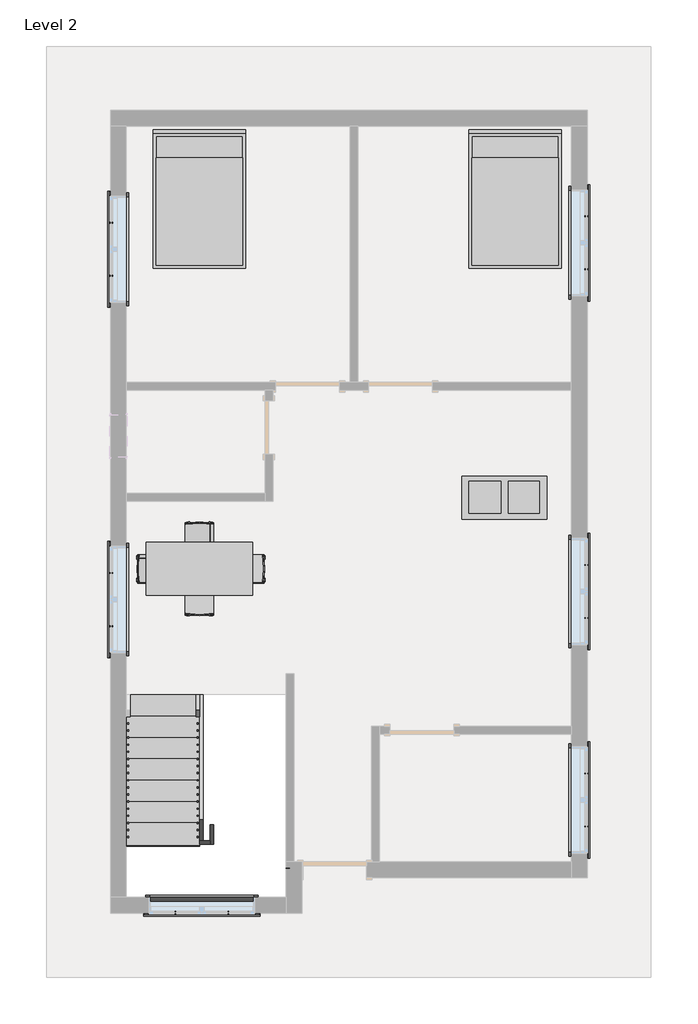
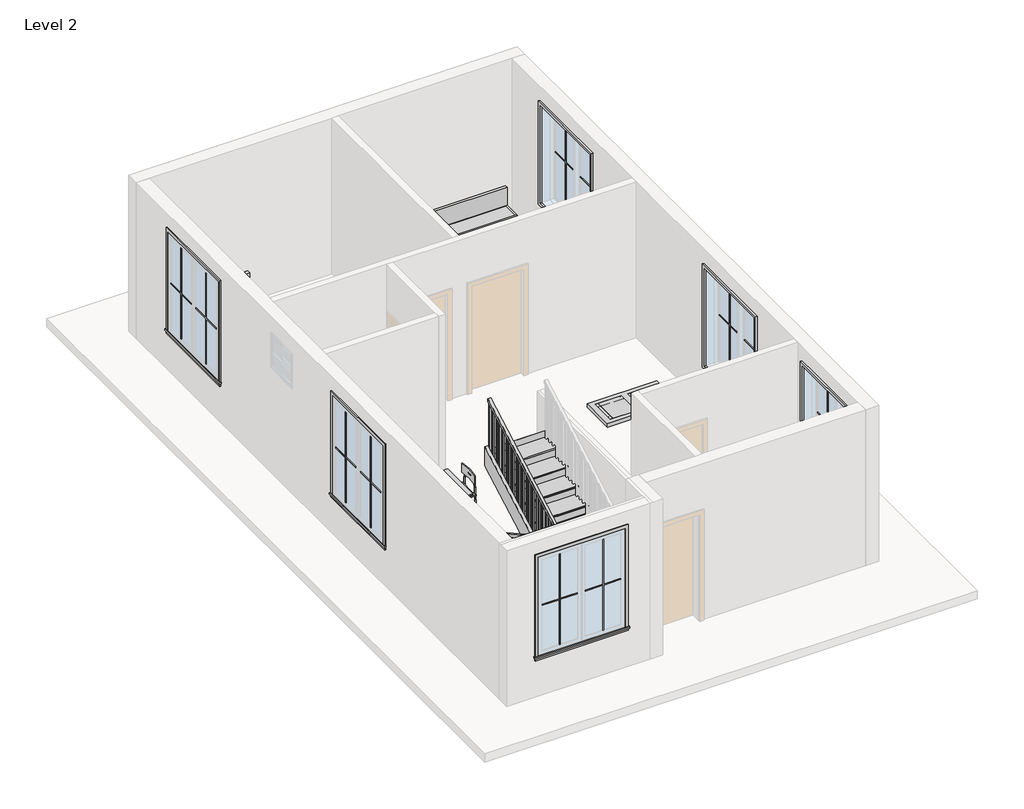
# One storey, part 3 of 3: 25 proxies, 6 members, 3 furniture elements, 1 railing, 1 stair flight.
"""IFC4 building model written with IfcOpenShell, lengths in millimetres."""

from ifc_helpers import new_model, si_unit, frame, origin, place, context, project, spatial, polyline, outline, extrude, faceted_brep, transform, mapped, element, save
from components import muntin_pattern_2x2_muntin_pattern_2x2_f6a80940, muntin_pattern_2x2_muntin_pattern_2x2_09b00a1c, trim_window_exterior_flat_with_sill_698ed857, trim_window_interior_flat_picture_frame_92551a5e, coffee_table_with_brass_mullions_11320_coffee_table_with_5962bef7, bed_17739_bed_17739_15c61121, dining_table_w_chairs_11374_0cdfc61b, stair_flight_d5b1d6b9

model = new_model("IFC4")

# Units and contexts
model_context = context("Model", 3, world=origin())
ifc_project = project(units=[si_unit("LENGTHUNIT", "METRE", prefix="MILLI")], contexts=[model_context])

# Site, building, storey
site = spatial("IfcSite", under=ifc_project)
building = spatial("IfcBuilding", under=site)
storey = spatial("IfcBuildingStorey", under=building, Name="Level 2", Elevation=3048.0)

# Proxies
placement = place(None, origin())
muntin_pattern_2x2_muntin_pattern_2x2_shape = muntin_pattern_2x2_muntin_pattern_2x2_f6a80940(model_context)
element("IfcBuildingElementProxy", 1, Name="Muntin Pattern_2x2 : Muntin Pattern_2x2", ObjectType="Muntin Pattern_2x2 : Muntin Pattern_2x2", at=placement, inside=storey, context=model_context, shape_type="MappedRepresentation", body=[
    mapped(muntin_pattern_2x2_muntin_pattern_2x2_shape, transform((-2773.368364, -6686.2830018, 4032.25), x_axis=(-1.0, 0.0, 0.0), y_axis=(0.0, -1.0, 0.0), z_axis=(0.0, 0.0, 1.0))),
])
element("IfcBuildingElementProxy", 2, Name="Muntin Pattern_2x2 : Muntin Pattern_2x2", ObjectType="Muntin Pattern_2x2 : Muntin Pattern_2x2", at=placement, inside=storey, context=model_context, shape_type="MappedRepresentation", body=[
    mapped(muntin_pattern_2x2_muntin_pattern_2x2_shape, transform((2349.494136, -4693.9705018, 4032.25), x_axis=(0.0, -1.0, 0.0), y_axis=(1.0, 0.0, 0.0), z_axis=(0.0, 0.0, 1.0))),
])
element("IfcBuildingElementProxy", 3, Name="Muntin Pattern_2x2 : Muntin Pattern_2x2", ObjectType="Muntin Pattern_2x2 : Muntin Pattern_2x2", at=placement, inside=storey, context=model_context, shape_type="MappedRepresentation", body=[
    mapped(muntin_pattern_2x2_muntin_pattern_2x2_shape, transform((2349.494136, -1712.6455018, 4032.25), x_axis=(0.0, -1.0, 0.0), y_axis=(1.0, 0.0, 0.0), z_axis=(0.0, 0.0, 1.0))),
])
element("IfcBuildingElementProxy", 4, Name="Muntin Pattern_2x2 : Muntin Pattern_2x2", ObjectType="Muntin Pattern_2x2 : Muntin Pattern_2x2", at=placement, inside=storey, context=model_context, shape_type="MappedRepresentation", body=[
    mapped(muntin_pattern_2x2_muntin_pattern_2x2_shape, transform((-4451.355864, -2586.5525081, 4032.25), x_axis=(0.0, 1.0, 0.0), y_axis=(-1.0, 0.0, 0.0), z_axis=(0.0, 0.0, 1.0))),
])
element("IfcBuildingElementProxy", 5, Name="Muntin Pattern_2x2 : Muntin Pattern_2x2", ObjectType="Muntin Pattern_2x2 : Muntin Pattern_2x2", at=placement, inside=storey, context=model_context, shape_type="MappedRepresentation", body=[
    mapped(muntin_pattern_2x2_muntin_pattern_2x2_shape, transform((2349.494136, 3272.1044982, 4032.25), x_axis=(0.0, -1.0, 0.0), y_axis=(1.0, 0.0, 0.0), z_axis=(0.0, 0.0, 1.0))),
])
element("IfcBuildingElementProxy", 6, Name="Muntin Pattern_2x2 : Muntin Pattern_2x2", ObjectType="Muntin Pattern_2x2 : Muntin Pattern_2x2", at=placement, inside=storey, context=model_context, shape_type="MappedRepresentation", body=[
    mapped(muntin_pattern_2x2_muntin_pattern_2x2_shape, transform((-4451.355864, 2421.2162133, 4032.25), x_axis=(0.0, 1.0, 0.0), y_axis=(-1.0, 0.0, 0.0), z_axis=(0.0, 0.0, 1.0))),
])
muntin_pattern_2x2_muntin_pattern_2x2_2_shape = muntin_pattern_2x2_muntin_pattern_2x2_09b00a1c(model_context)
element("IfcBuildingElementProxy", 7, Name="Muntin Pattern_2x2 : Muntin Pattern_2x2", ObjectType="Muntin Pattern_2x2 : Muntin Pattern_2x2", at=placement, inside=storey, context=model_context, shape_type="MappedRepresentation", body=[
    mapped(muntin_pattern_2x2_muntin_pattern_2x2_2_shape, transform((-3532.193364, -6686.2830018, 4032.25), x_axis=(1.0, 0.0, 0.0), y_axis=(0.0, 1.0, 0.0), z_axis=(0.0, 0.0, 1.0))),
])
element("IfcBuildingElementProxy", 8, Name="Muntin Pattern_2x2 : Muntin Pattern_2x2", ObjectType="Muntin Pattern_2x2 : Muntin Pattern_2x2", at=placement, inside=storey, context=model_context, shape_type="MappedRepresentation", body=[
    mapped(muntin_pattern_2x2_muntin_pattern_2x2_2_shape, transform((2349.494136, -5452.7955018, 4032.25), x_axis=(0.0, 1.0, 0.0), y_axis=(-1.0, 0.0, 0.0), z_axis=(0.0, 0.0, 1.0))),
])
element("IfcBuildingElementProxy", 9, Name="Muntin Pattern_2x2 : Muntin Pattern_2x2", ObjectType="Muntin Pattern_2x2 : Muntin Pattern_2x2", at=placement, inside=storey, context=model_context, shape_type="MappedRepresentation", body=[
    mapped(muntin_pattern_2x2_muntin_pattern_2x2_2_shape, transform((2349.494136, -2471.4705018, 4032.25), x_axis=(0.0, 1.0, 0.0), y_axis=(-1.0, 0.0, 0.0), z_axis=(0.0, 0.0, 1.0))),
])
element("IfcBuildingElementProxy", 10, Name="Muntin Pattern_2x2 : Muntin Pattern_2x2", ObjectType="Muntin Pattern_2x2 : Muntin Pattern_2x2", at=placement, inside=storey, context=model_context, shape_type="MappedRepresentation", body=[
    mapped(muntin_pattern_2x2_muntin_pattern_2x2_2_shape, transform((-4451.355864, -1827.7275081, 4032.25), x_axis=(0.0, -1.0, 0.0), y_axis=(1.0, 0.0, 0.0), z_axis=(0.0, 0.0, 1.0))),
])
element("IfcBuildingElementProxy", 11, Name="Muntin Pattern_2x2 : Muntin Pattern_2x2", ObjectType="Muntin Pattern_2x2 : Muntin Pattern_2x2", at=placement, inside=storey, context=model_context, shape_type="MappedRepresentation", body=[
    mapped(muntin_pattern_2x2_muntin_pattern_2x2_2_shape, transform((2349.494136, 2513.2794982, 4032.25), x_axis=(0.0, 1.0, 0.0), y_axis=(-1.0, 0.0, 0.0), z_axis=(0.0, 0.0, 1.0))),
])
element("IfcBuildingElementProxy", 12, Name="Muntin Pattern_2x2 : Muntin Pattern_2x2", ObjectType="Muntin Pattern_2x2 : Muntin Pattern_2x2", at=placement, inside=storey, context=model_context, shape_type="MappedRepresentation", body=[
    mapped(muntin_pattern_2x2_muntin_pattern_2x2_2_shape, transform((-4451.355864, 3180.0412133, 4032.25), x_axis=(0.0, -1.0, 0.0), y_axis=(1.0, 0.0, 0.0), z_axis=(0.0, 0.0, 1.0))),
])
trim_window_exterior_flat_with_sill_shape = trim_window_exterior_flat_with_sill_698ed857(model_context)
element("IfcBuildingElementProxy", 13, Name="Trim-Window-Exterior-Flat : with Sill", ObjectType="Trim-Window-Exterior-Flat : with Sill", at=placement, inside=storey, context=model_context, shape_type="MappedRepresentation", body=[
    mapped(trim_window_exterior_flat_with_sill_shape, transform((-3152.780864, -6695.8080018, 5791.2), x_axis=(1.0, 0.0, 0.0), y_axis=(0.0, 0.0, 1.0), z_axis=(0.0, -1.0, 0.0))),
])
element("IfcBuildingElementProxy", 14, Name="Trim-Window-Exterior-Flat : with Sill", ObjectType="Trim-Window-Exterior-Flat : with Sill", at=placement, inside=storey, context=model_context, shape_type="MappedRepresentation", body=[
    mapped(trim_window_exterior_flat_with_sill_shape, transform((2359.019136, -5073.3830018, 5791.2), x_axis=(0.0, 1.0, 0.0), y_axis=(0.0, 0.0, 1.0), z_axis=(1.0, 0.0, 0.0))),
])
element("IfcBuildingElementProxy", 15, Name="Trim-Window-Exterior-Flat : with Sill", ObjectType="Trim-Window-Exterior-Flat : with Sill", at=placement, inside=storey, context=model_context, shape_type="MappedRepresentation", body=[
    mapped(trim_window_exterior_flat_with_sill_shape, transform((2359.019136, -2092.0580018, 5791.2), x_axis=(0.0, 1.0, 0.0), y_axis=(0.0, 0.0, 1.0), z_axis=(1.0, 0.0, 0.0))),
])
element("IfcBuildingElementProxy", 16, Name="Trim-Window-Exterior-Flat : with Sill", ObjectType="Trim-Window-Exterior-Flat : with Sill", at=placement, inside=storey, context=model_context, shape_type="MappedRepresentation", body=[
    mapped(trim_window_exterior_flat_with_sill_shape, transform((-4460.880864, -2207.1400081, 5791.2), x_axis=(0.0, -1.0, 0.0), y_axis=(0.0, 0.0, 1.0), z_axis=(-1.0, 0.0, 0.0))),
])
element("IfcBuildingElementProxy", 17, Name="Trim-Window-Exterior-Flat : with Sill", ObjectType="Trim-Window-Exterior-Flat : with Sill", at=placement, inside=storey, context=model_context, shape_type="MappedRepresentation", body=[
    mapped(trim_window_exterior_flat_with_sill_shape, transform((2359.019136, 2892.6919982, 5791.2), x_axis=(0.0, 1.0, 0.0), y_axis=(0.0, 0.0, 1.0), z_axis=(1.0, 0.0, 0.0))),
])
element("IfcBuildingElementProxy", 18, Name="Trim-Window-Exterior-Flat : with Sill", ObjectType="Trim-Window-Exterior-Flat : with Sill", at=placement, inside=storey, context=model_context, shape_type="MappedRepresentation", body=[
    mapped(trim_window_exterior_flat_with_sill_shape, transform((-4460.880864, 2800.6287133, 5791.2), x_axis=(0.0, -1.0, 0.0), y_axis=(0.0, 0.0, 1.0), z_axis=(-1.0, 0.0, 0.0))),
])
trim_window_interior_flat_picture_frame_shape = trim_window_interior_flat_picture_frame_92551a5e(model_context)
element("IfcBuildingElementProxy", 19, Name="Trim-Window-Interior-Flat : Picture Frame", ObjectType="Trim-Window-Interior-Flat : Picture Frame", at=placement, inside=storey, context=model_context, shape_type="MappedRepresentation", body=[
    mapped(trim_window_interior_flat_picture_frame_shape, transform((-3152.780864, -6467.2080018, 5791.2), x_axis=(-1.0, 0.0, 0.0), y_axis=(0.0, 0.0, 1.0), z_axis=(0.0, 1.0, 0.0))),
])
element("IfcBuildingElementProxy", 20, Name="Trim-Window-Interior-Flat : Picture Frame", ObjectType="Trim-Window-Interior-Flat : Picture Frame", at=placement, inside=storey, context=model_context, shape_type="MappedRepresentation", body=[
    mapped(trim_window_interior_flat_picture_frame_shape, transform((2130.419136, -5073.3830018, 5791.2), x_axis=(0.0, -1.0, 0.0), y_axis=(0.0, 0.0, 1.0), z_axis=(-1.0, 0.0, 0.0))),
])
element("IfcBuildingElementProxy", 21, Name="Trim-Window-Interior-Flat : Picture Frame", ObjectType="Trim-Window-Interior-Flat : Picture Frame", at=placement, inside=storey, context=model_context, shape_type="MappedRepresentation", body=[
    mapped(trim_window_interior_flat_picture_frame_shape, transform((2130.419136, -2092.0580018, 5791.2), x_axis=(0.0, -1.0, 0.0), y_axis=(0.0, 0.0, 1.0), z_axis=(-1.0, 0.0, 0.0))),
])
element("IfcBuildingElementProxy", 22, Name="Trim-Window-Interior-Flat : Picture Frame", ObjectType="Trim-Window-Interior-Flat : Picture Frame", at=placement, inside=storey, context=model_context, shape_type="MappedRepresentation", body=[
    mapped(trim_window_interior_flat_picture_frame_shape, transform((-4232.280864, -2207.1400081, 5791.2), x_axis=(0.0, 1.0, 0.0), y_axis=(0.0, 0.0, 1.0), z_axis=(1.0, 0.0, 0.0))),
])
element("IfcBuildingElementProxy", 23, Name="Trim-Window-Interior-Flat : Picture Frame", ObjectType="Trim-Window-Interior-Flat : Picture Frame", at=placement, inside=storey, context=model_context, shape_type="MappedRepresentation", body=[
    mapped(trim_window_interior_flat_picture_frame_shape, transform((2130.419136, 2892.6919982, 5791.2), x_axis=(0.0, -1.0, 0.0), y_axis=(0.0, 0.0, 1.0), z_axis=(-1.0, 0.0, 0.0))),
])
element("IfcBuildingElementProxy", 24, Name="Trim-Window-Interior-Flat : Picture Frame", ObjectType="Trim-Window-Interior-Flat : Picture Frame", at=placement, inside=storey, context=model_context, shape_type="MappedRepresentation", body=[
    mapped(trim_window_interior_flat_picture_frame_shape, transform((-4232.280864, 2800.6287133, 5791.2), x_axis=(0.0, 1.0, 0.0), y_axis=(0.0, 0.0, 1.0), z_axis=(1.0, 0.0, 0.0))),
])
coffee_table_with_brass_mullions_11320_coffee_table_with_shape = coffee_table_with_brass_mullions_11320_coffee_table_with_5962bef7(model_context)
element("IfcBuildingElementProxy", 25, Name="coffee_table_with_brass_mullions_11320 : coffee_table_with_brass_mullions_11320", ObjectType="coffee_table_with_brass_mullions_11320 : coffee_table_with_brass_mullions_11320", at=placement, inside=storey, context=model_context, shape_type="MappedRepresentation", body=[
    mapped(coffee_table_with_brass_mullions_11320_coffee_table_with_shape, transform((1812.3816081, -1181.1001099, 3048.0), x_axis=(1.0, 0.0, 0.0), y_axis=(0.0, 1.0, 0.0), z_axis=(0.0, 0.0, 1.0))),
])

# Furniture
bed_17739_bed_17739_shape = bed_17739_bed_17739_15c61121(model_context)
element("IfcFurniture", 26, ObjectType="Bed_17739 : Bed_17739", at=placement, inside=storey, context=model_context, shape_type="MappedRepresentation", body=[
    mapped(bed_17739_bed_17739_shape, transform((1328.5116081, 3496.3098901, 3048.0), x_axis=(1.0, 0.0, 0.0), y_axis=(0.0, 1.0, 0.0), z_axis=(0.0, 0.0, 1.0))),
])
element("IfcFurniture", 27, ObjectType="Bed_17739 : Bed_17739", at=placement, inside=storey, context=model_context, shape_type="MappedRepresentation", body=[
    mapped(bed_17739_bed_17739_shape, transform((-3187.6083919, 3496.3098901, 3048.0), x_axis=(1.0, 0.0, 0.0), y_axis=(0.0, 1.0, 0.0), z_axis=(0.0, 0.0, 1.0))),
])
dining_table_w_chairs_11374_shape = dining_table_w_chairs_11374_0cdfc61b(model_context)
element("IfcFurniture", 28, ObjectType="Dining_Table_w_Chairs_11374", at=placement, inside=storey, context=model_context, shape_type="MappedRepresentation", body=[
    mapped(dining_table_w_chairs_11374_shape, transform((-3205.8741586, -1863.0511877, 3048.0), x_axis=(1.0, 0.0, 0.0), y_axis=(0.0, 1.0, 0.0), z_axis=(0.0, 0.0, 1.0))),
])

# Members
element("IfcMember", 29, ObjectType="Stringer - 2\" Width", at=placement, inside=storey, context=model_context, shape_type="SweptSolid", body=[
    extrude(outline(polyline([(-3571.6080018, 3255.5983948), (-3571.6080018, 3048.0), (-3825.5525046, 3048.0), (-5654.4080018, 4064.0308318), (-5654.4080018, 4412.7095059), (-3571.6080018, 3255.5983948)])), frame((-3187.6083919, 0.0, 0.0), z_axis=(1.0, 0.0, 0.0), x_axis=(0.0, 1.0, 0.0)), (0.0, 0.0, 1.0), 50.8),
])
element("IfcMember", 30, ObjectType="Stringer - 2\" Width", at=placement, inside=storey, context=model_context, shape_type="SweptSolid", body=[
    extrude(outline(polyline([(-3187.6083919, -5705.2080018), (-3187.6083919, -5654.4080018), (-3035.2083919, -5654.4080018), (-3035.2083919, -5705.2080018), (-3187.6083919, -5705.2080018)])), frame((0.0, 0.0, 4174.0666667), z_axis=(0.0, 0.0, 1.0), x_axis=(1.0, 0.0, 0.0)), (0.0, 0.0, 1.0), 304.8),
])
element("IfcMember", 31, ObjectType="Stringer - 2\" Width", at=placement, inside=storey, context=model_context, shape_type="SweptSolid", body=[
    extrude(outline(polyline([(-5705.2080018, 4174.0666667), (-5705.2080018, 4440.9317281), (-3571.6080018, 5626.2650614), (-3571.6080018, 5277.5863873), (-5557.943499, 4174.0666667), (-5705.2080018, 4174.0666667)])), frame((-3035.2083919, 0.0, 0.0), z_axis=(1.0, 0.0, 0.0), x_axis=(0.0, 1.0, 0.0)), (0.0, 0.0, 1.0), 50.8),
])
element("IfcMember", 32, ObjectType="Stringer - 2\" Width", at=placement, inside=storey, context=model_context, shape_type="SweptSolid", body=[
    extrude(outline(polyline([(-3571.6080018, 3255.5983948), (-3571.6080018, 3048.0), (-3825.5525046, 3048.0), (-6401.1125046, 4478.8666667), (-5773.4908912, 4478.8666667), (-3571.6080018, 3255.5983948)])), frame((-4283.080864, 0.0, 0.0), z_axis=(1.0, 0.0, 0.0), x_axis=(0.0, 1.0, 0.0)), (0.0, 0.0, 1.0), 50.8),
])
element("IfcMember", 33, ObjectType="Stringer - 2\" Width", at=placement, inside=storey, context=model_context, shape_type="SweptSolid", body=[
    extrude(outline(polyline([(-4283.080864, -6518.0080018), (-4283.080864, -6467.2080018), (-1946.280864, -6467.2080018), (-1946.280864, -6518.0080018), (-4283.080864, -6518.0080018)])), frame((0.0, 0.0, 4174.0666667), z_axis=(0.0, 0.0, 1.0), x_axis=(1.0, 0.0, 0.0)), (0.0, 0.0, 1.0), 304.8),
])
element("IfcMember", 34, ObjectType="Stringer - 2\" Width", at=placement, inside=storey, context=model_context, shape_type="SweptSolid", body=[
    extrude(outline(polyline([(-6185.5651124, 4174.0666667), (-3571.6080018, 5626.2650614), (-3571.6080018, 5277.5863873), (-5557.943499, 4174.0666667), (-6185.5651124, 4174.0666667)])), frame((-1946.280864, 0.0, 0.0), z_axis=(1.0, 0.0, 0.0), x_axis=(0.0, 1.0, 0.0)), (0.0, 0.0, 1.0), 50.8),
])

# Railing
element("IfcRailing", 35, ObjectType="Handrail - Rectangular", at=placement, inside=storey, context=model_context, shape_type="SolidModel", body=[
    faceted_brep([(-3187.6083919, -3571.6080018, 4131.7333333), (-3187.6083919, -3571.6080018, 4073.620221), (-3238.4083919, -3571.6080018, 4073.620221), (-3238.4083919, -3571.6080018, 4131.7333333), (-3187.6083919, -5629.0080018, 5274.7333333), (-3187.6083919, -5679.8080018, 5244.8424432), (-3238.4083919, -5679.8080018, 5244.8424432), (-3238.4083919, -5629.0080018, 5274.7333333), (-3187.6083919, -5629.0080018, 5317.0666667), (-3187.6083919, -5679.8080018, 5266.2666667), (-3238.4083919, -5679.8080018, 5266.2666667), (-3238.4083919, -5629.0080018, 5317.0666667), (-3187.6083919, -5705.2080018, 5317.0666667), (-3187.6083919, -5705.2080018, 5266.2666667), (-3238.4083919, -5756.0080018, 5266.2666667), (-3238.4083919, -5756.0080018, 5317.0666667), (-3111.4083919, -5705.2080018, 5317.0666667), (-3111.4083919, -5705.2080018, 5266.2666667), (-3111.4083919, -5756.0080018, 5266.2666667), (-3111.4083919, -5756.0080018, 5317.0666667), (-3060.6083919, -5705.2080018, 5317.0666667), (-3009.8083919, -5705.2080018, 5266.2666667), (-3009.8083919, -5756.0080018, 5266.2666667), (-3060.6083919, -5756.0080018, 5317.0666667), (-3060.6083919, -5705.2080018, 5359.4), (-3009.8083919, -5705.2080018, 5308.6), (-3009.8083919, -5756.0080018, 5308.6), (-3060.6083919, -5756.0080018, 5359.4), (-2984.4083919, -5705.2080018, 5359.4), (-2984.4083919, -5705.2080018, 5308.6), (-2933.6083919, -5756.0080018, 5308.6), (-2933.6083919, -5756.0080018, 5359.4), (-2984.4083919, -5629.0080018, 5359.4), (-2984.4083919, -5615.8443995, 5308.6), (-2933.6083919, -5615.8443995, 5308.6), (-2933.6083919, -5629.0080018, 5359.4), (-2984.4083919, -3571.6080018, 6502.4), (-2933.6083919, -3571.6080018, 6502.4), (-2933.6083919, -3571.6080018, 6444.2868876), (-2984.4083919, -3571.6080018, 6444.2868876)], [[[0, 1, 2, 3]], [[1, 0, 4, 5]], [[2, 1, 5, 6]], [[3, 2, 6, 7]], [[0, 3, 7, 4]], [[5, 4, 8, 9]], [[6, 5, 9, 10]], [[7, 6, 10, 11]], [[4, 7, 11, 8]], [[9, 8, 12, 13]], [[10, 9, 13, 14]], [[11, 10, 14, 15]], [[8, 11, 15, 12]], [[13, 12, 16, 17]], [[14, 13, 17, 18]], [[15, 14, 18, 19]], [[12, 15, 19, 16]], [[17, 16, 20, 21]], [[18, 17, 21, 22]], [[19, 18, 22, 23]], [[16, 19, 23, 20]], [[21, 20, 24, 25]], [[22, 21, 25, 26]], [[23, 22, 26, 27]], [[20, 23, 27, 24]], [[25, 24, 28, 29]], [[26, 25, 29, 30]], [[27, 26, 30, 31]], [[24, 27, 31, 28]], [[29, 28, 32, 33]], [[30, 29, 33, 34]], [[31, 30, 34, 35]], [[28, 31, 35, 32]], [[36, 37, 38, 39]], [[33, 32, 36, 39]], [[34, 33, 39, 38]], [[35, 34, 38, 37]], [[32, 35, 37, 36]]]),
    extrude(outline(polyline([(-3587.4830018, 6435.4674432), (-3587.4830018, 5418.6666667), (-3606.5330018, 5418.6666667), (-3606.5330018, 6424.8841099), (-3587.4830018, 6435.4674432)])), frame((-2968.5333919, 0.0, 0.0), z_axis=(1.0, 0.0, 0.0), x_axis=(0.0, 1.0, 0.0)), (0.0, 0.0, 1.0), 19.05),
    extrude(outline(polyline([(-3689.0830018, 6379.0229988), (-3689.0830018, 5418.6666667), (-3708.1330018, 5418.6666667), (-3708.1330018, 6368.4396654), (-3689.0830018, 6379.0229988)])), frame((-2968.5333919, 0.0, 0.0), z_axis=(1.0, 0.0, 0.0), x_axis=(0.0, 1.0, 0.0)), (0.0, 0.0, 1.0), 19.05),
    extrude(outline(polyline([(-3790.6830018, 6322.5785543), (-3790.6830018, 5418.6666667), (-3809.7330018, 5418.6666667), (-3809.7330018, 6311.995221), (-3790.6830018, 6322.5785543)])), frame((-2968.5333919, 0.0, 0.0), z_axis=(1.0, 0.0, 0.0), x_axis=(0.0, 1.0, 0.0)), (0.0, 0.0, 1.0), 19.05),
    extrude(outline(polyline([(-3892.2830018, 6266.1341099), (-3892.2830018, 5249.3333333), (-3911.3330018, 5249.3333333), (-3911.3330018, 6255.5507765), (-3892.2830018, 6266.1341099)])), frame((-2968.5333919, 0.0, 0.0), z_axis=(1.0, 0.0, 0.0), x_axis=(0.0, 1.0, 0.0)), (0.0, 0.0, 1.0), 19.05),
    extrude(outline(polyline([(-3993.8830018, 6209.6896654), (-3993.8830018, 5249.3333333), (-4012.9330018, 5249.3333333), (-4012.9330018, 6199.1063321), (-3993.8830018, 6209.6896654)])), frame((-2968.5333919, 0.0, 0.0), z_axis=(1.0, 0.0, 0.0), x_axis=(0.0, 1.0, 0.0)), (0.0, 0.0, 1.0), 19.05),
    extrude(outline(polyline([(-4095.4830018, 6153.245221), (-4095.4830018, 5249.3333333), (-4114.5330018, 5249.3333333), (-4114.5330018, 6142.6618876), (-4095.4830018, 6153.245221)])), frame((-2968.5333919, 0.0, 0.0), z_axis=(1.0, 0.0, 0.0), x_axis=(0.0, 1.0, 0.0)), (0.0, 0.0, 1.0), 19.05),
    extrude(outline(polyline([(-4197.0830018, 6096.8007765), (-4197.0830018, 5080.0), (-4216.1330018, 5080.0), (-4216.1330018, 6086.2174432), (-4197.0830018, 6096.8007765)])), frame((-2968.5333919, 0.0, 0.0), z_axis=(1.0, 0.0, 0.0), x_axis=(0.0, 1.0, 0.0)), (0.0, 0.0, 1.0), 19.05),
    extrude(outline(polyline([(-4298.6830018, 6040.3563321), (-4298.6830018, 5080.0), (-4317.7330018, 5080.0), (-4317.7330018, 6029.7729988), (-4298.6830018, 6040.3563321)])), frame((-2968.5333919, 0.0, 0.0), z_axis=(1.0, 0.0, 0.0), x_axis=(0.0, 1.0, 0.0)), (0.0, 0.0, 1.0), 19.05),
    extrude(outline(polyline([(-4400.2830018, 5983.9118876), (-4400.2830018, 5080.0), (-4419.3330018, 5080.0), (-4419.3330018, 5973.3285543), (-4400.2830018, 5983.9118876)])), frame((-2968.5333919, 0.0, 0.0), z_axis=(1.0, 0.0, 0.0), x_axis=(0.0, 1.0, 0.0)), (0.0, 0.0, 1.0), 19.05),
    extrude(outline(polyline([(-4501.8830018, 5927.4674432), (-4501.8830018, 4910.6666667), (-4520.9330018, 4910.6666667), (-4520.9330018, 5916.8841099), (-4501.8830018, 5927.4674432)])), frame((-2968.5333919, 0.0, 0.0), z_axis=(1.0, 0.0, 0.0), x_axis=(0.0, 1.0, 0.0)), (0.0, 0.0, 1.0), 19.05),
    extrude(outline(polyline([(-4603.4830018, 5871.0229988), (-4603.4830018, 4910.6666667), (-4622.5330018, 4910.6666667), (-4622.5330018, 5860.4396654), (-4603.4830018, 5871.0229988)])), frame((-2968.5333919, 0.0, 0.0), z_axis=(1.0, 0.0, 0.0), x_axis=(0.0, 1.0, 0.0)), (0.0, 0.0, 1.0), 19.05),
    extrude(outline(polyline([(-4705.0830018, 5814.5785543), (-4705.0830018, 4910.6666667), (-4724.1330018, 4910.6666667), (-4724.1330018, 5803.995221), (-4705.0830018, 5814.5785543)])), frame((-2968.5333919, 0.0, 0.0), z_axis=(1.0, 0.0, 0.0), x_axis=(0.0, 1.0, 0.0)), (0.0, 0.0, 1.0), 19.05),
    extrude(outline(polyline([(-4806.6830018, 5758.1341099), (-4806.6830018, 4741.3333333), (-4825.7330018, 4741.3333333), (-4825.7330018, 5747.5507765), (-4806.6830018, 5758.1341099)])), frame((-2968.5333919, 0.0, 0.0), z_axis=(1.0, 0.0, 0.0), x_axis=(0.0, 1.0, 0.0)), (0.0, 0.0, 1.0), 19.05),
    extrude(outline(polyline([(-4908.2830018, 5701.6896654), (-4908.2830018, 4741.3333333), (-4927.3330018, 4741.3333333), (-4927.3330018, 5691.1063321), (-4908.2830018, 5701.6896654)])), frame((-2968.5333919, 0.0, 0.0), z_axis=(1.0, 0.0, 0.0), x_axis=(0.0, 1.0, 0.0)), (0.0, 0.0, 1.0), 19.05),
    extrude(outline(polyline([(-5009.8830018, 5645.245221), (-5009.8830018, 4741.3333333), (-5028.9330018, 4741.3333333), (-5028.9330018, 5634.6618876), (-5009.8830018, 5645.245221)])), frame((-2968.5333919, 0.0, 0.0), z_axis=(1.0, 0.0, 0.0), x_axis=(0.0, 1.0, 0.0)), (0.0, 0.0, 1.0), 19.05),
    extrude(outline(polyline([(-5111.4830018, 5588.8007765), (-5111.4830018, 4572.0), (-5130.5330018, 4572.0), (-5130.5330018, 5578.2174432), (-5111.4830018, 5588.8007765)])), frame((-2968.5333919, 0.0, 0.0), z_axis=(1.0, 0.0, 0.0), x_axis=(0.0, 1.0, 0.0)), (0.0, 0.0, 1.0), 19.05),
    extrude(outline(polyline([(-5213.0830018, 5532.3563321), (-5213.0830018, 4572.0), (-5232.1330018, 4572.0), (-5232.1330018, 5521.7729988), (-5213.0830018, 5532.3563321)])), frame((-2968.5333919, 0.0, 0.0), z_axis=(1.0, 0.0, 0.0), x_axis=(0.0, 1.0, 0.0)), (0.0, 0.0, 1.0), 19.05),
    extrude(outline(polyline([(-5314.6830018, 5475.9118876), (-5314.6830018, 4572.0), (-5333.7330018, 4572.0), (-5333.7330018, 5465.3285543), (-5314.6830018, 5475.9118876)])), frame((-2968.5333919, 0.0, 0.0), z_axis=(1.0, 0.0, 0.0), x_axis=(0.0, 1.0, 0.0)), (0.0, 0.0, 1.0), 19.05),
    extrude(outline(polyline([(-5416.2830018, 5419.4674432), (-5416.2830018, 4402.6666667), (-5435.3330018, 4402.6666667), (-5435.3330018, 5408.8841099), (-5416.2830018, 5419.4674432)])), frame((-2968.5333919, 0.0, 0.0), z_axis=(1.0, 0.0, 0.0), x_axis=(0.0, 1.0, 0.0)), (0.0, 0.0, 1.0), 19.05),
    extrude(outline(polyline([(-5517.8830018, 5363.0229988), (-5517.8830018, 4402.6666667), (-5536.9330018, 4402.6666667), (-5536.9330018, 5352.4396654), (-5517.8830018, 5363.0229988)])), frame((-2968.5333919, 0.0, 0.0), z_axis=(1.0, 0.0, 0.0), x_axis=(0.0, 1.0, 0.0)), (0.0, 0.0, 1.0), 19.05),
    extrude(outline(polyline([(-5619.4830018, 5306.5785543), (-5619.4830018, 4402.6666667), (-5638.5330018, 4402.6666667), (-5638.5330018, 5295.995221), (-5619.4830018, 5306.5785543)])), frame((-2968.5333919, 0.0, 0.0), z_axis=(1.0, 0.0, 0.0), x_axis=(0.0, 1.0, 0.0)), (0.0, 0.0, 1.0), 19.05),
    extrude(outline(polyline([(-3019.3333919, -5721.0830018), (-3000.2833919, -5721.0830018), (-3000.2833919, -5740.1330018), (-3019.3333919, -5740.1330018), (-3019.3333919, -5721.0830018)])), frame((0.0, 0.0, 4402.6666667), z_axis=(0.0, 0.0, 1.0), x_axis=(1.0, 0.0, 0.0)), (0.0, 0.0, 1.0), 905.9333333),
    extrude(outline(polyline([(-3120.9333919, -5721.0830018), (-3101.8833919, -5721.0830018), (-3101.8833919, -5740.1330018), (-3120.9333919, -5740.1330018), (-3120.9333919, -5721.0830018)])), frame((0.0, 0.0, 4402.6666667), z_axis=(0.0, 0.0, 1.0), x_axis=(1.0, 0.0, 0.0)), (0.0, 0.0, 1.0), 863.6),
    extrude(outline(polyline([(-3203.4833919, -5695.6830018), (-3203.4833919, -5714.7330018), (-3222.5333919, -5714.7330018), (-3222.5333919, -5695.6830018), (-3203.4833919, -5695.6830018)])), frame((0.0, 0.0, 4402.6666667), z_axis=(0.0, 0.0, 1.0), x_axis=(1.0, 0.0, 0.0)), (0.0, 0.0, 1.0), 863.6),
    extrude(outline(polyline([(-5594.0830018, 5197.2174432), (-5594.0830018, 4233.3333333), (-5613.1330018, 4233.3333333), (-5613.1330018, 5207.8007765), (-5594.0830018, 5197.2174432)])), frame((-3222.5333919, 0.0, 0.0), z_axis=(1.0, 0.0, 0.0), x_axis=(0.0, 1.0, 0.0)), (0.0, 0.0, 1.0), 19.05),
    extrude(outline(polyline([(-5492.4830018, 5140.7729988), (-5492.4830018, 4233.3333333), (-5511.5330018, 4233.3333333), (-5511.5330018, 5151.3563321), (-5492.4830018, 5140.7729988)])), frame((-3222.5333919, 0.0, 0.0), z_axis=(1.0, 0.0, 0.0), x_axis=(0.0, 1.0, 0.0)), (0.0, 0.0, 1.0), 19.05),
    extrude(outline(polyline([(-5390.8830018, 5084.3285543), (-5390.8830018, 4233.3333333), (-5409.9330018, 4233.3333333), (-5409.9330018, 5094.9118876), (-5390.8830018, 5084.3285543)])), frame((-3222.5333919, 0.0, 0.0), z_axis=(1.0, 0.0, 0.0), x_axis=(0.0, 1.0, 0.0)), (0.0, 0.0, 1.0), 19.05),
    extrude(outline(polyline([(-5289.2830018, 5027.8841099), (-5289.2830018, 4064.0), (-5308.3330018, 4064.0), (-5308.3330018, 5038.4674432), (-5289.2830018, 5027.8841099)])), frame((-3222.5333919, 0.0, 0.0), z_axis=(1.0, 0.0, 0.0), x_axis=(0.0, 1.0, 0.0)), (0.0, 0.0, 1.0), 19.05),
    extrude(outline(polyline([(-5187.6830018, 4971.4396654), (-5187.6830018, 4064.0), (-5206.7330018, 4064.0), (-5206.7330018, 4982.0229988), (-5187.6830018, 4971.4396654)])), frame((-3222.5333919, 0.0, 0.0), z_axis=(1.0, 0.0, 0.0), x_axis=(0.0, 1.0, 0.0)), (0.0, 0.0, 1.0), 19.05),
    extrude(outline(polyline([(-5086.0830018, 4914.995221), (-5086.0830018, 4064.0), (-5105.1330018, 4064.0), (-5105.1330018, 4925.5785543), (-5086.0830018, 4914.995221)])), frame((-3222.5333919, 0.0, 0.0), z_axis=(1.0, 0.0, 0.0), x_axis=(0.0, 1.0, 0.0)), (0.0, 0.0, 1.0), 19.05),
    extrude(outline(polyline([(-4984.4830018, 4858.5507765), (-4984.4830018, 3894.6666667), (-5003.5330018, 3894.6666667), (-5003.5330018, 4869.1341099), (-4984.4830018, 4858.5507765)])), frame((-3222.5333919, 0.0, 0.0), z_axis=(1.0, 0.0, 0.0), x_axis=(0.0, 1.0, 0.0)), (0.0, 0.0, 1.0), 19.05),
    extrude(outline(polyline([(-4882.8830018, 4802.1063321), (-4882.8830018, 3894.6666667), (-4901.9330018, 3894.6666667), (-4901.9330018, 4812.6896654), (-4882.8830018, 4802.1063321)])), frame((-3222.5333919, 0.0, 0.0), z_axis=(1.0, 0.0, 0.0), x_axis=(0.0, 1.0, 0.0)), (0.0, 0.0, 1.0), 19.05),
    extrude(outline(polyline([(-4781.2830018, 4745.6618876), (-4781.2830018, 3894.6666667), (-4800.3330018, 3894.6666667), (-4800.3330018, 4756.245221), (-4781.2830018, 4745.6618876)])), frame((-3222.5333919, 0.0, 0.0), z_axis=(1.0, 0.0, 0.0), x_axis=(0.0, 1.0, 0.0)), (0.0, 0.0, 1.0), 19.05),
    extrude(outline(polyline([(-4679.6830018, 4689.2174432), (-4679.6830018, 3725.3333333), (-4698.7330018, 3725.3333333), (-4698.7330018, 4699.8007765), (-4679.6830018, 4689.2174432)])), frame((-3222.5333919, 0.0, 0.0), z_axis=(1.0, 0.0, 0.0), x_axis=(0.0, 1.0, 0.0)), (0.0, 0.0, 1.0), 19.05),
    extrude(outline(polyline([(-4578.0830018, 4632.7729988), (-4578.0830018, 3725.3333333), (-4597.1330018, 3725.3333333), (-4597.1330018, 4643.3563321), (-4578.0830018, 4632.7729988)])), frame((-3222.5333919, 0.0, 0.0), z_axis=(1.0, 0.0, 0.0), x_axis=(0.0, 1.0, 0.0)), (0.0, 0.0, 1.0), 19.05),
    extrude(outline(polyline([(-4476.4830018, 4576.3285543), (-4476.4830018, 3725.3333333), (-4495.5330018, 3725.3333333), (-4495.5330018, 4586.9118876), (-4476.4830018, 4576.3285543)])), frame((-3222.5333919, 0.0, 0.0), z_axis=(1.0, 0.0, 0.0), x_axis=(0.0, 1.0, 0.0)), (0.0, 0.0, 1.0), 19.05),
    extrude(outline(polyline([(-4374.8830018, 4519.8841099), (-4374.8830018, 3556.0), (-4393.9330018, 3556.0), (-4393.9330018, 4530.4674432), (-4374.8830018, 4519.8841099)])), frame((-3222.5333919, 0.0, 0.0), z_axis=(1.0, 0.0, 0.0), x_axis=(0.0, 1.0, 0.0)), (0.0, 0.0, 1.0), 19.05),
    extrude(outline(polyline([(-4273.2830018, 4463.4396654), (-4273.2830018, 3556.0), (-4292.3330018, 3556.0), (-4292.3330018, 4474.0229988), (-4273.2830018, 4463.4396654)])), frame((-3222.5333919, 0.0, 0.0), z_axis=(1.0, 0.0, 0.0), x_axis=(0.0, 1.0, 0.0)), (0.0, 0.0, 1.0), 19.05),
    extrude(outline(polyline([(-4171.6830018, 4406.995221), (-4171.6830018, 3556.0), (-4190.7330018, 3556.0), (-4190.7330018, 4417.5785543), (-4171.6830018, 4406.995221)])), frame((-3222.5333919, 0.0, 0.0), z_axis=(1.0, 0.0, 0.0), x_axis=(0.0, 1.0, 0.0)), (0.0, 0.0, 1.0), 19.05),
    extrude(outline(polyline([(-4070.0830018, 4350.5507765), (-4070.0830018, 3386.6666667), (-4089.1330018, 3386.6666667), (-4089.1330018, 4361.1341099), (-4070.0830018, 4350.5507765)])), frame((-3222.5333919, 0.0, 0.0), z_axis=(1.0, 0.0, 0.0), x_axis=(0.0, 1.0, 0.0)), (0.0, 0.0, 1.0), 19.05),
    extrude(outline(polyline([(-3968.4830018, 4294.1063321), (-3968.4830018, 3386.6666667), (-3987.5330018, 3386.6666667), (-3987.5330018, 4304.6896654), (-3968.4830018, 4294.1063321)])), frame((-3222.5333919, 0.0, 0.0), z_axis=(1.0, 0.0, 0.0), x_axis=(0.0, 1.0, 0.0)), (0.0, 0.0, 1.0), 19.05),
    extrude(outline(polyline([(-3866.8830018, 4237.6618876), (-3866.8830018, 3386.6666667), (-3885.9330018, 3386.6666667), (-3885.9330018, 4248.245221), (-3866.8830018, 4237.6618876)])), frame((-3222.5333919, 0.0, 0.0), z_axis=(1.0, 0.0, 0.0), x_axis=(0.0, 1.0, 0.0)), (0.0, 0.0, 1.0), 19.05),
    extrude(outline(polyline([(-3765.2830018, 4181.2174432), (-3765.2830018, 3217.3333333), (-3784.3330018, 3217.3333333), (-3784.3330018, 4191.8007765), (-3765.2830018, 4181.2174432)])), frame((-3222.5333919, 0.0, 0.0), z_axis=(1.0, 0.0, 0.0), x_axis=(0.0, 1.0, 0.0)), (0.0, 0.0, 1.0), 19.05),
    extrude(outline(polyline([(-3663.6830018, 4124.7729988), (-3663.6830018, 3217.3333333), (-3682.7330018, 3217.3333333), (-3682.7330018, 4135.3563321), (-3663.6830018, 4124.7729988)])), frame((-3222.5333919, 0.0, 0.0), z_axis=(1.0, 0.0, 0.0), x_axis=(0.0, 1.0, 0.0)), (0.0, 0.0, 1.0), 19.05),
    extrude(outline(polyline([(-2968.5333919, -5721.0830018), (-2949.4833919, -5721.0830018), (-2949.4833919, -5740.1330018), (-2968.5333919, -5740.1330018), (-2968.5333919, -5721.0830018)])), frame((0.0, 0.0, 4402.6666667), z_axis=(0.0, 0.0, 1.0), x_axis=(1.0, 0.0, 0.0)), (0.0, 0.0, 1.0), 905.9333333),
    extrude(outline(polyline([(-3203.4833919, -5721.0830018), (-3203.4833919, -5740.1330018), (-3222.5333919, -5740.1330018), (-3222.5333919, -5721.0830018), (-3203.4833919, -5721.0830018)])), frame((0.0, 0.0, 4402.6666667), z_axis=(0.0, 0.0, 1.0), x_axis=(1.0, 0.0, 0.0)), (0.0, 0.0, 1.0), 863.6),
    extrude(outline(polyline([(-3571.6080018, 6444.2868876), (-3571.6080018, 5418.6666667), (-3590.6580018, 5418.6666667), (-3590.6580018, 6433.7035543), (-3571.6080018, 6444.2868876)])), frame((-2968.5333919, 0.0, 0.0), z_axis=(1.0, 0.0, 0.0), x_axis=(0.0, 1.0, 0.0)), (0.0, 0.0, 1.0), 19.05),
    extrude(outline(polyline([(-3571.6080018, 4073.620221), (-3571.6080018, 3217.3333333), (-3590.6580018, 3217.3333333), (-3590.6580018, 4084.2035543), (-3571.6080018, 4073.620221)])), frame((-3222.5333919, 0.0, 0.0), z_axis=(1.0, 0.0, 0.0), x_axis=(0.0, 1.0, 0.0)), (0.0, 0.0, 1.0), 19.05),
])

# Stair flight
stair_flight_shape = stair_flight_d5b1d6b9(model_context)
element("IfcStairFlight", 36, ObjectType="2\" Tread 1\" Nosing 1/4\" Riser", at=placement, inside=storey, context=model_context, shape_type="MappedRepresentation", body=[
    mapped(stair_flight_shape, transform((0.0, 0.0, 0.0), x_axis=(1.0, 0.0, 0.0), y_axis=(0.0, 1.0, 0.0), z_axis=(0.0, 0.0, 1.0))),
])

save(model, "model.ifc")

# Revit data of these elements
# Type "Muntin Pattern_2x2 : Muntin Pattern_2x2"
#   Width [instance default] = 4' - 0"
#   Thickness = 0' - 0 1/2"
#   Height [instance default] = 4' - 0"
#   Distance = 0' - 0 3/4"
#   Interior Material [instance default] = none
#   Exterior Material [instance default] = none
#   Default Elevation = 0
# Type "Trim-Window-Exterior-Flat : with Sill"
#   Trim Width = 0' - 2 1/4"
#   Trim Thickness_Picture Frame = 0' - 1 1/4"
#   Trim Thickness_with Sill = 0' - 0 3/4"
#   Sill Thickness = 0' - 1 1/4"
#   Opening Width [instance default] = 2' - 0"
#   Opening Height [instance default] = 3' - 0"
#   Default Elevation = 4' - 0"
#   Sill = yes
#   Picture Frame = no
#   Trim Material [instance default] = none
# Type "Trim-Window-Interior-Flat : Picture Frame"
#   Trim Thickness_Picture Frame = 0' - 1 1/4"
#   Trim Width = 0' - 2 1/4"
#   Trim Thickness_with Sill = 0' - 0 3/4"
#   Sill Thickness = 0' - 1 1/4"
#   Opening Width [instance default] = 2' - 0"
#   Opening Height [instance default] = 3' - 0"
#   Default Elevation = 4' - 0"
#   Sill = no
#   Picture Frame = yes
#   Trim Material [instance default] = none
# Type "coffee_table_with_brass_mullions_11320 : coffee_table_with_brass_mullions_11320"
#   Default Elevation = 0
# Type "Bed_17739 : Bed_17739"
#   Default Elevation = 0
# Type "Dining_Table_w_Chairs_11374"
#   Default Elevation = 0
#   Assembly Code = ""
# Type "Handrail - Rectangular"
#   Assembly Code = "C2010400"
#   built-in parameter 1008612 = 0.0416667 (stored number, unit not read)
#   built-in parameter 1008611 = 0.0416667 (stored number, unit not read)
#   built-in parameter 1008609 = 0.333333 (stored number, unit not read)
#   built-in parameter 1008604 = 0.166667 (stored number, unit not read)
#   built-in parameter 1008603 = 0.166667 (stored number, unit not read)
#   Railing Height = 3' - 0"
#   built-in parameter 1008630 = 2
#   built-in parameter 1008610 = 2
#   built-in parameter 1008618 = Baluster - Square : 3/4"
# Elements 1, 2, 3, 4, 5, 6, 7, 8, 9, 10, 11, 12 (IfcBuildingElementProxy, "Muntin Pattern_2x2 : Muntin Pattern_2x2")
#   Width = 2' - 0 5/8"
#   Height = 5' - 6 1/2"
#   Interior Material = Wood - Stained
#   Exterior Material = Clad - White
#   Phase Created = New Construction
#   Materials on its faces: "Clad - White", "Wood - Stained"
# Elements 13, 14, 15, 16, 17, 18 (IfcBuildingElementProxy, "Trim-Window-Exterior-Flat : with Sill")
#   Opening Width = 5' - 0"
#   Opening Height = 6' - 0"
#   Trim Material = Clad - White
#   Phase Created = New Construction
#   Materials on its faces: "Clad - White"
# Elements 19, 20, 21, 22, 23, 24 (IfcBuildingElementProxy, "Trim-Window-Interior-Flat : Picture Frame")
#   Opening Width = 5' - 0"
#   Opening Height = 6' - 0"
#   Trim Material = Wood - Stained
#   Phase Created = New Construction
#   Materials on its faces: "Wood - Stained"
# Element 25 (IfcBuildingElementProxy, "coffee_table_with_brass_mullions_11320 : coffee_table_with_brass_mullions_11320")
#   Phase Created = New Construction
#   Materials on its faces: "Default Wall", "TABLE", "Glass", "Default"
# Elements 26, 27 (IfcFurniture, "Bed_17739 : Bed_17739")
#   Phase Created = New Construction
#   Materials on its faces: "legs", "sheets", "bed frame", "Blanket"
# Element 28 (IfcFurniture, "Dining_Table_w_Chairs_11374")
#   Phase Created = New Construction
# Elements 29, 30, 31, 32, 33, 34 (IfcMember, "Stringer - 2\" Width")
#   Phase Created = New Construction
# Element 35 (IfcRailing, "Handrail - Rectangular")
#   Phase Created = New Construction
# Element 36 (IfcStairFlight, "2\" Tread 1\" Nosing 1/4\" Riser")
#   Phase Created = New Construction
# Materials
#   "Clad - White": class "Wood", colour RGB 242 242 238, transparency 0, Cost = 0
#   "Wood - Stained": class "Wood", colour RGB 224 178 126, transparency 0, Cost = 0
#   "Default Wall": colour RGB 128 128 128, transparency 0, Cost = 0
#   "TABLE": class "Generic", colour RGB 120 120 120, transparency 0, Cost = 0
#   "Glass": class "Glass", colour RGB 0 128 192, transparency 0.75, Description = "Soda Lime Glass", Cost = 0
#   "Default": colour RGB 127 127 127, transparency 0, Cost = 0
#   "legs": colour RGB 90 73 37, transparency 0, Cost = 0
#   "sheets": colour RGB 200 195 176, transparency 0, Cost = 0
#   "bed frame": colour RGB 90 73 37, transparency 0, Cost = 0
#   "Blanket": class "System", colour RGB 59 0 1, transparency 0, Cost = 0
